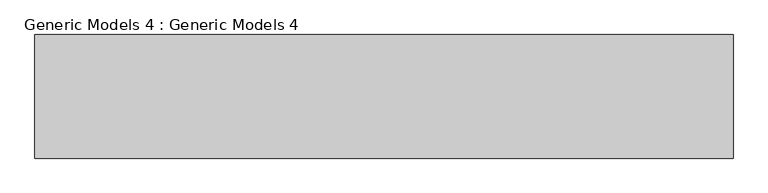
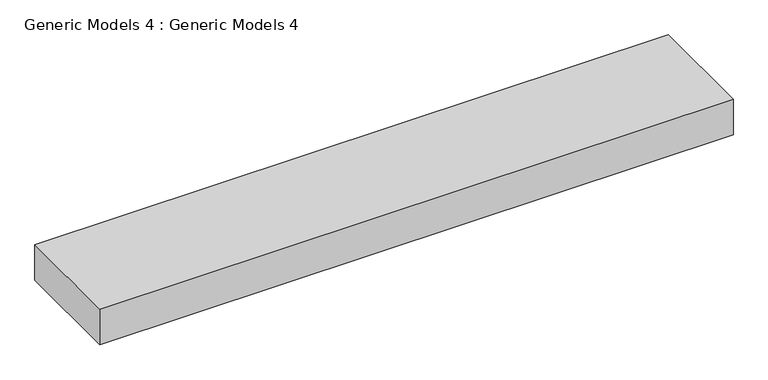
"""IFC4 building model written with IfcOpenShell, lengths in millimetres: proxy geometry, Generic Models 4 : Generic Models 4."""

from ifc_helpers import new_model, si_unit, frame, origin, place, context, project, spatial, polyline, outline, extrude, source, transform, mapped, element, save


def generic_models_4_generic_models_4_6b078398(model_context):
    return source(origin(), model_context, "Body", "SweptSolid", [
        extrude(outline(polyline([(-25335.3977446, -16327.2030397), (-25335.3977446, -12718.8007309), (-4957.034663, -12718.8007309), (-4957.034663, -16327.2030397), (-25335.3977446, -16327.2030397)])), frame((0.0, 0.0, 59056.089321), z_axis=(0.0, 0.0, 1.0), x_axis=(1.0, 0.0, 0.0)), (0.0, 0.0, 1.0), 1215.737857),
    ])


if __name__ == "__main__":
    model = new_model("IFC4")
    model_context = context("Model", 3, world=origin())
    ifc_project = project(units=[si_unit("LENGTHUNIT", "METRE", prefix="MILLI")], contexts=[model_context])
    site = spatial("IfcSite", under=ifc_project)
    building = spatial("IfcBuilding", under=site)
    placement = place(None, origin())
    generic_models_4_generic_models_4_shape = generic_models_4_generic_models_4_6b078398(model_context)
    element("IfcBuildingElementProxy", 1, Name="Generic Models 4 : Generic Models 4", ObjectType="Generic Models 4 : Generic Models 4", at=placement, inside=building, context=model_context, shape_type="MappedRepresentation", body=[
        mapped(generic_models_4_generic_models_4_shape, transform((0.0, 0.0, 0.0), x_axis=(1.0, 0.0, 0.0), y_axis=(0.0, 1.0, 0.0), z_axis=(0.0, 0.0, 1.0))),
    ])
    save(model, "model.ifc")
